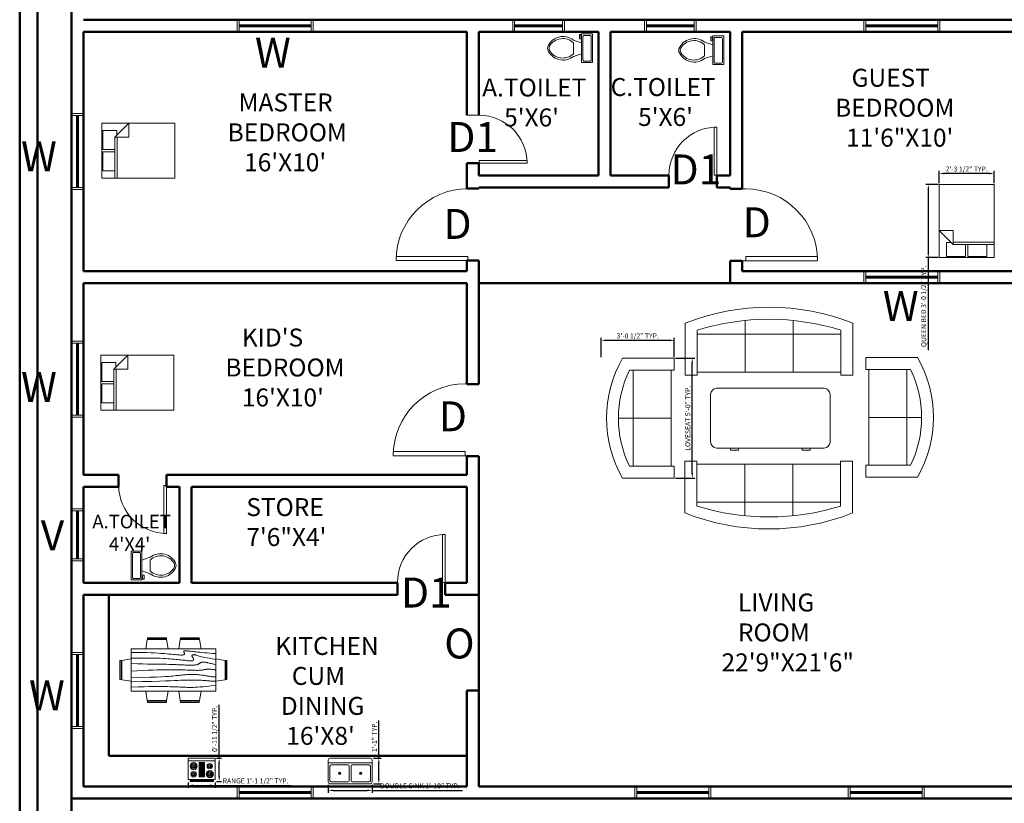
# Model space of a CAD drawing. Units: inches. Extents: x -7040 to -4088, y 6092 to 7645.
# Tile 4 of 11: x -7003 to -6510, y 6471 to 6864. Entities that reach past the tile are written whole.
import ezdxf

# ---------------------------------------------------------------- set-up
doc = ezdxf.new("R2010")
doc.units = ezdxf.units.IN
for name, color, linetype, lineweight in [('A-ANNO-DIMS', 2, 'Continuous', 18), ('A-ANNO-TEXT', 7, 'Continuous', 25), ('A-AREA-IDEN', 3, 'Continuous', 25), ('A-DOOR', 3, 'Continuous', 18), ('A-FLOR-FIXT', 9, 'Continuous', 13), ('A-FURN', 8, 'Continuous', 13), ('A-GLAZ', 4, 'Continuous', 18), ('A-WALL', 7, 'Continuous', 50)]:
    doc.layers.add(name, color=color, linetype=linetype, lineweight=lineweight)
doc.styles.get("Standard").update_dxf_attribs({"font": 'arial.ttf'})
doc.dimstyles.new('ISO-25', dxfattribs={"dimtxt": 2.5, "dimasz": 2.5, "dimexe": 1.25, "dimexo": 0.625, "dimtad": 1, "dimdec": 0, "dimlunit": 3, "dimtxsty": 'Standard', "dimcen": 2.5, "dimadec": 0, "dimazin": 0, "dimtfac": 1, "dimtdec": 0, "dimtmove": 0, "dimatfit": 3, "dimfxl": 1, "dimarcsym": 0})

# ---------------------------------------------------------------- blocks, each defined once
blk = doc.blocks.new('*U8')
for p, q in [((0, 0), (0, -100)), ((750, 0), (750, -100))]:
    blk.add_line(p, q)
blk.add_lwpolyline([(0, 0), (0, 750), (43.75, 750), (43.75, 0)], close=True)
blk.add_arc((0, 0), 750, 0, 90)
blk = doc.blocks.new('Bed - Queen')
for p, q in [((0, -80.00003), (0, 0)), ((0, 0), (59.99999, 0)), ((59.99999, 0), (59.99999, -80.00003)), ((7.99999, -1.2), (28.79998, -1.2)), ((7.99999, -14.4), (7.99999, -1.2)), ((28.79998, -1.2), (28.79998, -14.4)), ((31.19999, -1.2), (51.99999, -1.2)), ((31.19999, -14.4), (31.19999, -1.2)), ((51.99999, -1.2), (51.99999, -16.4)), ((0, -14.4), (44.8, -14.4)), ((44.8, -16.8), (0, -16.8)), ((59.99999, -29.6), (44.8, -14.4)), ((44.8, -14.4), (44.8, -29.6)), ((51.99999, -16.4), (46.79936, -16.4)), ((44.8, -29.6), (59.99999, -29.6)), ((59.99999, -80.00003), (0, -80.00003))]:
    blk.add_line(p, q)
blk = doc.blocks.new('Dining Set - 36 x 72 in.')
for p, q in [((-22.2343, 26.00059), (-23.4847, 17.99762)), ((-22.2304, 26), (-5.7608, 26)), ((-22, 27.5), (-22.1562, 26.50042)), ((-5.8416, 26.5), (-22.1534, 26.5)), ((-22, 27.5), (-6, 27.5)), ((-5.8437, 26.49966), (-6, 27.5)), ((-4.5152, 17.99762), (-5.7655, 25.99926)), ((5.7657, 26.00059), (4.5153, 17.99762)), ((5.7696, 26), (22.2392, 26)), ((6, 27.5), (5.8438, 26.50042)), ((22.1584, 26.5), (5.8466, 26.5)), ((6, 27.5), (22, 27.5)), ((22.1563, 26.49966), (22, 27.5)), ((23.4848, 17.99762), (22.2345, 25.99926)), ((36, 18), (-36, 18)), ((-36, 18), (-36, -18)), ((36, -18), (36, 18)), ((-44.0006, 8.23428), (-35.9976, 9.48474)), ((44.0006, 8.23428), (35.9976, 9.48474)), ((-45.5, 8), (-44.5004, 8.15617)), ((-45.5, 8), (-45.5, -8)), ((-44.5, -8.15843), (-44.5, 8.15338)), ((-44, 8.23041), (-44, -8.23915)), ((44, 8.23041), (44, -8.23915)), ((44.5, -8.15843), (44.5, 8.15338)), ((45.5, 8), (44.5005, 8.15617)), ((45.5, 8), (45.5, -8)), ((-44.4997, -8.15631), (-45.5, -8)), ((-35.9976, -9.48476), (-43.9993, -8.2345)), ((35.9976, -9.48476), (43.9993, -8.2345)), ((44.4997, -8.15631), (45.5, -8)), ((-36, -18), (36, -18)), ((-22.2343, -26.0006), (-23.4847, -17.99762)), ((-4.5152, -17.99762), (-5.7655, -25.99928)), ((5.7657, -26.0006), (4.5153, -17.99762)), ((23.4848, -17.99762), (22.2345, -25.99928)), ((-22.2304, -26), (-5.7608, -26)), ((-22, -27.5), (-22.1562, -26.50044)), ((-5.8416, -26.5), (-22.1534, -26.5)), ((-22, -27.5), (-6, -27.5)), ((-5.8437, -26.49967), (-6, -27.5)), ((5.7696, -26), (22.2392, -26)), ((6, -27.5), (5.8438, -26.50044)), ((22.1584, -26.5), (5.8466, -26.5)), ((6, -27.5), (22, -27.5)), ((22.1563, -26.49967), (22, -27.5))]:
    blk.add_line(p, q)
for points in [[(-36, 15), (-31.1772, 14.97754), (-26.8079, 14.91406), (-22.8538, 14.81543), (-19.276, 14.6875), (-16.0362, 14.53613), (-13.0957, 14.36718), (-10.4159, 14.18652), (-7.9583, 14), (-5.6904, 13.81315), (-3.6035, 13.63021), (-1.6954, 13.45508), (0.0365, 13.29166), (1.5945, 13.14388), (2.9811, 13.01562), (4.1988, 12.9108), (5.25, 12.83333), (6.1393, 12.78613), (6.8802, 12.76823), (7.4883, 12.77767), (7.9792, 12.8125), (8.3685, 12.87077), (8.6719, 12.95052), (8.9049, 13.0498), (9.0833, 13.16666), (9.2205, 13.29899), (9.3216, 13.44401), (9.3895, 13.59879), (9.4271, 13.76041), (9.4373, 13.92594), (9.4232, 14.09245), (9.3875, 14.257), (9.3333, 14.41666), (9.2638, 14.56917), (9.1836, 14.71484), (9.0975, 14.85465), (9.0104, 14.98958), (8.9272, 15.1206), (8.8529, 15.2487), (8.7922, 15.37483), (8.75, 15.5), (8.7305, 15.62467), (8.7344, 15.74739), (8.7617, 15.86621), (8.8125, 15.97916), (8.8867, 16.08431), (8.9844, 16.17968), (9.1055, 16.26334), (9.25, 16.33333), (9.4189, 16.38802), (9.6172, 16.42708), (9.8506, 16.45052), (10.125, 16.45833), (10.4463, 16.45052), (10.8203, 16.42708), (11.2529, 16.38802), (11.75, 16.33333), (12.3184, 16.26318), (12.9694, 16.17838), (13.7151, 16.07991), (14.5677, 15.96875), (15.5395, 15.84586), (16.6426, 15.71224), (17.8893, 15.56884), (19.2917, 15.41666), (20.859, 15.25667), (22.5879, 15.08984), (24.4721, 14.91715), (26.5052, 14.73958), (28.6809, 14.5581), (30.9929, 14.3737), (33.4347, 14.18733), (36, 14)], [(-36, 10), (-28.9766, 10.14274), (-23.1725, 10.20442), (-18.4241, 10.19775), (-14.5677, 10.13541), (-11.4399, 10.03011), (-8.877, 9.89453), (-6.7154, 9.74137), (-4.7917, 9.58333), (-2.9698, 9.43082), (-1.2246, 9.28515), (0.4415, 9.14534), (2.026, 9.01041), (3.5266, 8.87939), (4.9408, 8.7513), (6.266, 8.62516), (7.5, 8.5), (8.6411, 8.37549), (9.6914, 8.2539), (10.6538, 8.13818), (11.5312, 8.03125), (12.3267, 7.93603), (13.043, 7.85547), (13.6831, 7.79248), (14.25, 7.75), (14.7471, 7.7303), (15.1797, 7.73307), (15.5537, 7.75732), (15.875, 7.80208), (16.1494, 7.86637), (16.3828, 7.94922), (16.5811, 8.04964), (16.75, 8.16666), (16.8944, 8.29915), (17.0143, 8.44531), (17.1089, 8.60319), (17.1771, 8.77083), (17.218, 8.94629), (17.2305, 9.1276), (17.2137, 9.31282), (17.1667, 9.5), (17.0895, 9.6875), (16.987, 9.875), (16.8649, 10.0625), (16.7292, 10.25), (16.5856, 10.4375), (16.4401, 10.625), (16.2985, 10.8125), (16.1667, 11), (16.05, 11.18733), (15.9518, 11.3737), (15.8752, 11.5581), (15.8229, 11.73958), (15.798, 11.91715), (15.8034, 12.08984), (15.842, 12.25667), (15.9167, 12.41666), (16.0295, 12.56836), (16.1784, 12.70833), (16.3605, 12.83268), (16.5729, 12.9375), (16.8127, 13.01888), (17.0768, 13.07291), (17.3625, 13.0957), (17.6667, 13.08333), (17.9894, 13.03312), (18.3418, 12.94726), (18.7382, 12.82918), (19.1927, 12.68229), (19.7195, 12.51001), (20.3327, 12.31575), (21.0465, 12.10294), (21.875, 11.875), (22.8357, 11.63354), (23.959, 11.37304), (25.2786, 11.08618), (26.8282, 10.76562), (28.6414, 10.40405), (30.752, 9.99414), (33.1936, 9.52856), (36, 9)], [(-36, 5.5), (-30.7157, 5.3348), (-26.069, 5.20963), (-21.9946, 5.11767), (-18.4271, 5.05208), (-15.3009, 5.00602), (-12.5508, 4.97265), (-10.1112, 4.94515), (-7.9167, 4.91666), (-5.909, 4.88167), (-4.0586, 4.83984), (-2.3429, 4.79215), (-0.7396, 4.73958), (0.7739, 4.6831), (2.22, 4.6237), (3.6213, 4.56233), (5, 4.5), (6.373, 4.43782), (7.7344, 4.3776), (9.0723, 4.32129), (10.375, 4.27083), (11.6309, 4.22819), (12.8281, 4.19531), (13.9551, 4.17415), (15, 4.16666), (15.954, 4.17448), (16.819, 4.19791), (17.6001, 4.23698), (18.3021, 4.29166), (18.9299, 4.36198), (19.4883, 4.44791), (19.9823, 4.54948), (20.4167, 4.66666), (20.7969, 4.79899), (21.1302, 4.94401), (21.4245, 5.09879), (21.6875, 5.26041), (21.9271, 5.42594), (22.1511, 5.59245), (22.3672, 5.757), (22.5834, 5.91666), (22.8065, 6.06868), (23.0404, 6.21093), (23.2879, 6.34147), (23.5521, 6.45833), (23.8358, 6.55957), (24.142, 6.64323), (24.4735, 6.70735), (24.8334, 6.75), (25.2235, 6.76969), (25.642, 6.76692), (26.0858, 6.74267), (26.5521, 6.69791), (27.0379, 6.63362), (27.5404, 6.55078), (28.0565, 6.45036), (28.5834, 6.33333), (29.1242, 6.19987), (29.7071, 6.04687), (30.3661, 5.87044), (31.1354, 5.66666), (32.0493, 5.43164), (33.142, 5.16146), (34.4475, 4.85221), (36, 4.5)], [(-36, -1), (-30.7915, -0.6591), (-26.0195, -0.38216), (-21.6519, -0.16284), (-17.6563, 0.00521), (-14.0005, 0.12833), (-10.6523, 0.21289), (-7.5796, 0.26522), (-4.75, 0.29166), (-2.134, 0.29793), (0.2878, 0.28711), (2.5317, 0.26163), (4.6146, 0.22396), (6.5529, 0.17651), (8.3633, 0.12174), (10.0623, 0.06209), (11.6667, 0), (13.1899, -0.06201), (14.6341, -0.1211), (15.9982, -0.17432), (17.2813, -0.21875), (18.4823, -0.25147), (19.6003, -0.26953), (20.6343, -0.27002), (21.5834, -0.25), (22.4481, -0.20768), (23.2357, -0.14584), (23.9549, -0.06836), (24.6146, 0.02083), (25.2235, 0.11784), (25.7904, 0.21875), (26.3241, 0.31966), (26.8334, 0.41666), (27.3265, 0.50618), (27.8099, 0.58593), (28.2894, 0.65397), (28.7709, 0.70833), (29.2601, 0.74707), (29.763, 0.76823), (30.2855, 0.76985), (30.8334, 0.75), (31.4088, 0.70784), (31.9994, 0.64713), (32.589, 0.57275), (33.1615, 0.48958), (33.7008, 0.4025), (34.1908, 0.3164), (34.6153, 0.23616), (34.9584, 0.16666), (35.2099, 0.11165), (35.3848, 0.07031), (35.504, 0.04069), (35.5886, 0.02083), (35.6594, 0.00879), (35.7377, 0.0026), (35.8442, 0.00032), (36, 0)], [(-36, -6.5), (-27.1843, -6.31267), (-20.084, -6.1263), (-14.469, -5.9419), (-10.1094, -5.76042), (-6.7752, -5.58285), (-4.2363, -5.41016), (-2.2629, -5.24333), (-0.625, -5.08334), (0.8708, -4.93099), (2.2715, -4.78646), (3.5872, -4.64974), (4.8281, -4.52084), (6.0046, -4.39974), (7.127, -4.28646), (8.2053, -4.18099), (9.25, -4.08334), (10.2705, -3.99382), (11.2734, -3.91407), (12.2647, -3.84603), (13.25, -3.79167), (14.2354, -3.75293), (15.2266, -3.73177), (16.2295, -3.73015), (17.25, -3.75), (18.2912, -3.79248), (19.3451, -3.85547), (20.4009, -3.93604), (21.4479, -4.03125), (22.4754, -4.13819), (23.4727, -4.25391), (24.4289, -4.37549), (25.3334, -4.5), (26.1785, -4.62492), (26.9694, -4.74935), (27.7145, -4.87281), (28.4219, -4.99479), (29.1, -5.11483), (29.7572, -5.23242), (30.4016, -5.34709), (31.0417, -5.45834), (31.6837, -5.56437), (32.3262, -5.65821), (32.9658, -5.73153), (33.599, -5.77604), (34.2224, -5.78345), (34.8327, -5.74545), (35.4264, -5.65373), (36, -5.5)], [(-36, -10), (-26.4022, -9.81299), (-18.4675, -9.62891), (-11.9839, -9.45069), (-6.7396, -9.28125), (-2.5226, -9.12354), (0.8789, -8.98047), (3.6769, -8.85498), (6.0833, -8.75), (8.2767, -8.66765), (10.3021, -8.60677), (12.1712, -8.56543), (13.8958, -8.54167), (15.4876, -8.53353), (16.9583, -8.53907), (18.3197, -8.55632), (19.5834, -8.58334), (20.7616, -8.61841), (21.8685, -8.66081), (22.9188, -8.71004), (23.9271, -8.76563), (24.9081, -8.82707), (25.8763, -8.89388), (26.8465, -8.96558), (27.8334, -9.04167), (28.8474, -9.12118), (29.8828, -9.20117), (30.93, -9.27824), (31.9792, -9.34896), (33.0205, -9.40991), (34.0443, -9.45768), (35.0407, -9.48885), (36, -9.5)], [(-36, -14.5), (-30.0881, -14.33513), (-25.0332, -14.21224), (-20.7312, -14.12647), (-17.0781, -14.07292), (-13.97, -14.04671), (-11.3027, -14.04297), (-8.9724, -14.05681), (-6.875, -14.08334), (-4.9224, -14.11833), (-3.0905, -14.16016), (-1.3709, -14.20785), (0.2448, -14.26042), (1.7647, -14.3169), (3.1973, -14.3763), (4.5507, -14.43767), (5.8333, -14.5), (7.0554, -14.5621), (8.235, -14.62175), (9.3922, -14.67652), (10.5469, -14.72396), (11.7192, -14.76164), (12.929, -14.78711), (14.1965, -14.79794), (15.5417, -14.79167), (16.9933, -14.76424), (18.6152, -14.70508), (20.4804, -14.60197), (22.6615, -14.44271), (25.2312, -14.21509), (28.2624, -13.9069), (31.8277, -13.50594), (36, -13)]]:
    blk.add_lwpolyline(points)
blk = doc.blocks.new('Range-Oven - 30 in top')
for p, q in [((0, -3), (30, -3)), ((12, -6), (18, -6)), ((13, -20), (13, -6)), ((14, -6), (14, -20)), ((15, -20), (15, -6)), ((16, -6), (16, -20)), ((17, -20), (17, -6)), ((18, -20), (12, -20)), ((6, -24), (6, -25)), ((8, -25), (8, -24)), ((22, -25), (22, -24)), ((24, -24), (24, -25))]:
    blk.add_line(p, q)
for points in [[(0, -24), (0, 0), (30, 0), (30, -24)], [(12, -21), (12, -5), (18, -5), (18, -21)], [(2, -26), (2, -25), (28, -25), (28, -26)]]:
    blk.add_lwpolyline(points, close=True)
for centre, radius in [((6, -9), 4), ((6, -9), 3), ((6, -9), 2), ((6, -9), 1), ((24, -9), 3), ((24, -9), 2), ((24, -9), 1), ((6, -18), 3), ((6, -18), 2), ((6, -18), 1), ((24, -18), 4), ((24, -18), 3), ((24, -18), 2), ((24, -18), 1)]:
    blk.add_circle(centre, radius)
blk = doc.blocks.new('Sink-double - 36 in top')
for p, q in [((-18, -4), (18, -4)), ((-0.75, -18.5), (-0.75, -6.5)), ((0.75, -6.5), (0.75, -18.5))]:
    blk.add_line(p, q)
for points in [[(-16.5, 0), (16.5, 0)], [(-18, -19.5), (-18, -1.5)], [(-16.5, -18.5), (-16.5, -6.5)], [(-15.5, -5.5), (-1.75, -5.5)], [(1.75, -5.5), (15.5, -5.5)], [(16.5, -6.5), (16.5, -18.5)], [(18, -1.5), (18, -19.5)], [(16.5, -21), (-16.5, -21)], [(-1.75, -19.5), (-15.5, -19.5)], [(15.5, -19.5), (1.75, -19.5)]]:
    blk.add_lwpolyline(points)
for centre, radius in [((-8.5, -12.5), 1), ((-8.5, -12.5), 0.5), ((8.5, -12.5), 1), ((8.5, -12.5), 0.5)]:
    blk.add_circle(centre, radius)
for centre, radius, start, end in [((-16.5, -1.5), 1.5, 90, 180), ((16.5, -1.5), 1.5, 0, 90), ((-15.5, -6.5), 1, 90, 180), ((-1.75, -6.5), 1, 0, 90), ((1.75, -6.5), 1, 90, 180), ((15.5, -6.5), 1, 0, 90), ((-16.5, -19.5), 1.5, 180, 270), ((-15.5, -18.5), 1, 180, 270), ((-1.75, -18.5), 1, 270, 0), ((1.75, -18.5), 1, 180, 270), ((15.5, -18.5), 1, 270, 0), ((16.5, -19.5), 1.5, 270, 0)]:
    blk.add_arc(centre, radius, start, end)
blk = doc.blocks.new('Desk - 30 x 60 in.')
for p, q in [((-26.999995, 0), (26.999995, 0)), ((-29.999995, -27), (-29.999995, -3)), ((29.999995, -3), (29.999995, -27)), ((26.999995, -30), (-26.999995, -30)), ((-20.000005, -30), (-20.000005, -31)), ((-20.000005, -31), (-16.000005, -31)), ((-16.000005, -31), (-16.000005, -30)), ((15.999995, -31), (15.999995, -30)), ((19.999995, -31), (15.999995, -31)), ((19.999995, -30), (19.999995, -31))]:
    blk.add_line(p, q)
for centre, start, end in [((-26.499995, -3.5), 98.1301, 171.8699), ((26.499995, -3.5), 8.130102, 81.8699), ((-26.499995, -26.5), 188.1301, 261.8699), ((26.499995, -26.5), 278.1301, 351.8699)]:
    blk.add_arc(centre, 3.535534, start, end)
blk = doc.blocks.new('Sofa - Roundback 7 ft.')
for p, q in [((-12.00002, -32.4421), (-12.00003, -6.5971)), ((11.99997, -32.4421), (11.99998, -6.5971)), ((-36.000027, -34), (-36.000027, -11.4696)), ((-35.999844, -13.3819), (35.9998, -13.3819)), ((35.99998, -34), (35.99998, -11.4696)), ((-36.000027, -32.4421), (35.99998, -32.4421))]:
    blk.add_line(p, q)
for points in [[(-36.000027, -34), (-42.000027, -34), (-42.000027, -8)], [(41.99998, -8), (41.99998, -34), (35.99998, -34)]]:
    blk.add_lwpolyline(points)
for centre, radius, start, end in [((0, -114.25), 114.25, 68.43141, 111.5686), ((-0.00001, -127.1968), 121.1968, 72.72033, 107.2797)]:
    blk.add_arc(centre, radius, start, end)
blk = doc.blocks.new('Sofa - Roundback Loveseat 5 ft.')
for p, q in [((0, -32.44198), (0, -5.99998)), ((-24, -33.99998), (-24, -11.46958)), ((-23.9998, -13.38178), (23.99986, -13.38178)), ((24.00004, -33.99998), (24.00004, -11.46958)), ((-24, -32.44198), (24.00004, -32.44198))]:
    blk.add_line(p, q)
for points in [[(-24, -33.99998), (-30, -33.99998), (-30, -7.99998)], [(30.00004, -7.99998), (30.00004, -33.99998), (24.00004, -33.99998)]]:
    blk.add_lwpolyline(points)
for centre, radius, start, end in [((0, -60.24998), 60.24998, 60.13715, 119.8628), ((0, -61.38438), 55.38444, 64.32083, 115.6792)]:
    blk.add_arc(centre, radius, start, end)
blk = doc.blocks.new('Toilet - top')
for p, q in [((9.5, -6), (9.5, -2)), ((-10, -8.5), (-8, -8.5)), ((-10, -9.5), (-10, -8.5)), ((-7, -9.5), (-10, -9.5)), ((-8, -8.5), (-8, -8)), ((-7, -8), (-7, -9.5)), ((-4, -8), (-6, -14)), ((4, -14), (-4, -14)), ((4, -8), (6, -14))]:
    blk.add_line(p, q)
blk.add_lwpolyline([(10.5, -8), (10.5, 0), (-10.5, 0), (-10.5, -8)], close=True)
for points in [[(-9.5, -2), (-9.5, -6)], [(8.5, -1), (-8.5, -1)], [(-8.5, -7), (8.5, -7)]]:
    blk.add_lwpolyline(points)
for centre, radius, start, end in [((-8.62, -1.88), 0.884, 81.8699, 188.1301), ((-8.62, -6.12), 0.884, 171.8699, 278.1301), ((8.62, -1.88), 0.884, 351.8699, 98.1301), ((8.62, -6.12), 0.884, 261.8699, 8.1301), ((3.52, -21.58), 12.17, 141.46911, 247.97143), ((4.2, -21.82), 11.33, 136.36773, 238.94682), ((-3.52, -21.58), 12.17, 292.02843, 38.53071), ((-4.2, -21.82), 11.33, 301.05301, 43.63209), ((0, -27.88), 4, 245.73182, 294.26817), ((0, -29), 4, 254.86053, 285.13947)]:
    blk.add_arc(centre, radius, start, end)
blk = doc.blocks.new('WIN-36')
for p, q in [((0, 6), (0, 0)), ((1, 6), (1, 0)), ((37, 6), (37, 0)), ((38, 6), (38, 0)), ((1, 3.5), (37, 3.5)), ((1, 3), (37, 3)), ((1, 2.5), (37, 2.5))]:
    blk.add_line(p, q)
blk = doc.blocks.new('WIN-24')
for p, q in [((0, 6), (0, 0)), ((1, 6), (1, 0)), ((25, 6), (25, 0)), ((26, 6), (26, 0)), ((1, 3.5), (25, 3.5)), ((1, 3), (25, 3)), ((1, 2.5), (25, 2.5))]:
    blk.add_line(p, q)
blk = doc.blocks.new('*D122')
at = {"layer": 'A-ANNO-DIMS', "color": 0, "lineweight": -2, "transparency": 16777216}
for p, q in [((-6542.92, 6781.25), (-6549.04, 6781.25)), ((-6547.79, 6778.75), (-6547.79, 6747.1)), ((-6542.92, 6744.6), (-6549.04, 6744.6)), ((-6547.79, 6744.6), (-6547.79, 6698.25))]:
    blk.add_line(p, q, dxfattribs=at)
at = {"layer": 'A-ANNO-DIMS', "color": 0, "transparency": 16777216}
for points in [[(-6548.2, 6778.75), (-6547.37, 6778.75), (-6547.79, 6781.25)], [(-6548.2, 6747.1), (-6547.37, 6747.1), (-6547.79, 6744.6)]]:
    blk.add_solid(points, dxfattribs=at)
at = {"layer": 'Defpoints', "color": 0, "transparency": 16777216}
for p in [(-6542.29, 6781.25), (-6547.79, 6744.6), (-6542.29, 6744.6)]:
    blk.add_point(p, dxfattribs=at)
at = {"layer": 'A-ANNO-DIMS', "color": 0, "transparency": 16777216, "insert": (-6549.78, 6720.18), "char_height": 2.5, "attachment_point": 5, "rotation": 90}
blk.add_mtext('QUEEN BED 3\'-0 1/2" TYP.', dxfattribs=at)
blk = doc.blocks.new('*D123')
at = {"layer": 'A-ANNO-DIMS', "color": 0, "lineweight": -2, "transparency": 16777216}
for p, q in [((-6542.29, 6781.87), (-6542.29, 6787.99)), ((-6517.31, 6786.74), (-6539.79, 6786.74)), ((-6514.81, 6781.87), (-6514.81, 6787.99))]:
    blk.add_line(p, q, dxfattribs=at)
at = {"layer": 'A-ANNO-DIMS', "color": 0, "transparency": 16777216}
for points in [[(-6539.79, 6787.16), (-6539.79, 6786.33), (-6542.29, 6786.74)], [(-6517.31, 6787.16), (-6517.31, 6786.33), (-6514.81, 6786.74)]]:
    blk.add_solid(points, dxfattribs=at)
at = {"layer": 'Defpoints', "color": 0, "transparency": 16777216}
for p in [(-6542.29, 6786.74), (-6542.29, 6781.25), (-6514.81, 6781.25)]:
    blk.add_point(p, dxfattribs=at)
at = {"layer": 'A-ANNO-DIMS', "color": 0, "transparency": 16777216, "insert": (-6528.55, 6788.66), "char_height": 2.5, "attachment_point": 5}
blk.add_mtext('2\'-3 1/2" TYP.', dxfattribs=at)
blk = doc.blocks.new('*D134')
at = {"layer": 'A-ANNO-DIMS', "color": 0, "lineweight": -2, "transparency": 16777216}
for p, q in [((-6674.42, 6694.16), (-6664.79, 6694.16)), ((-6666.04, 6636.66), (-6666.04, 6691.66)), ((-6674.42, 6634.16), (-6664.79, 6634.16))]:
    blk.add_line(p, q, dxfattribs=at)
at = {"layer": 'A-ANNO-DIMS', "color": 0, "transparency": 16777216}
for points in [[(-6666.46, 6691.66), (-6665.62, 6691.66), (-6666.04, 6694.16)], [(-6666.46, 6636.66), (-6665.62, 6636.66), (-6666.04, 6634.16)]]:
    blk.add_solid(points, dxfattribs=at)
at = {"layer": 'Defpoints', "color": 0, "transparency": 16777216}
for p in [(-6675.04, 6694.16), (-6666.04, 6694.16), (-6675.04, 6634.16)]:
    blk.add_point(p, dxfattribs=at)
at = {"layer": 'A-ANNO-DIMS', "color": 0, "transparency": 16777216, "insert": (-6667.96, 6664.16), "char_height": 2.5, "attachment_point": 5, "rotation": 90}
blk.add_mtext('LOVESEAT 5\'-0" TYP.', dxfattribs=at)
blk = doc.blocks.new('*D135')
at = {"layer": 'A-ANNO-DIMS', "color": 0, "lineweight": -2, "transparency": 16777216}
for p, q in [((-6711.71, 6694.79), (-6711.71, 6704.41)), ((-6675.04, 6694.79), (-6675.04, 6704.41)), ((-6677.54, 6703.16), (-6709.21, 6703.16))]:
    blk.add_line(p, q, dxfattribs=at)
at = {"layer": 'A-ANNO-DIMS', "color": 0, "transparency": 16777216}
for points in [[(-6709.21, 6703.58), (-6709.21, 6702.74), (-6711.71, 6703.16)], [(-6677.54, 6703.58), (-6677.54, 6702.74), (-6675.04, 6703.16)]]:
    blk.add_solid(points, dxfattribs=at)
at = {"layer": 'Defpoints', "color": 0, "transparency": 16777216}
for p in [(-6711.71, 6703.16), (-6711.71, 6694.16), (-6675.04, 6694.16)]:
    blk.add_point(p, dxfattribs=at)
at = {"layer": 'A-ANNO-DIMS', "color": 0, "transparency": 16777216, "insert": (-6693.37, 6705.08), "char_height": 2.5, "attachment_point": 5}
blk.add_mtext('3\'-0 1/2" TYP.', dxfattribs=at)
blk = doc.blocks.new('*D148')
at = {"layer": 'A-ANNO-DIMS', "color": 0, "lineweight": -2, "transparency": 16777216}
for p, q in [((-6918.55, 6481.67), (-6918.55, 6479.03)), ((-6916.05, 6480.28), (-6907.61, 6480.28)), ((-6905.11, 6481.67), (-6905.11, 6479.03)), ((-6905.11, 6480.28), (-6867.04, 6480.28))]:
    blk.add_line(p, q, dxfattribs=at)
at = {"layer": 'A-ANNO-DIMS', "color": 0, "transparency": 16777216}
for points in [[(-6916.05, 6480.69), (-6916.05, 6479.86), (-6918.55, 6480.28)], [(-6907.61, 6480.69), (-6907.61, 6479.86), (-6905.11, 6480.28)]]:
    blk.add_solid(points, dxfattribs=at)
at = {"layer": 'Defpoints', "color": 0, "transparency": 16777216}
for p in [(-6918.55, 6482.29), (-6905.11, 6482.29), (-6905.11, 6480.28)]:
    blk.add_point(p, dxfattribs=at)
at = {"layer": 'A-ANNO-DIMS', "color": 0, "transparency": 16777216, "insert": (-6884.83, 6482.19), "char_height": 2.5, "attachment_point": 5}
blk.add_mtext('RANGE 1\'-1 1/2" TYP.', dxfattribs=at)
blk = doc.blocks.new('*D149')
at = {"layer": 'A-ANNO-DIMS', "color": 0, "lineweight": -2, "transparency": 16777216}
for p, q in [((-6903.1, 6493.94), (-6903.1, 6520.69)), ((-6904.49, 6493.94), (-6901.85, 6493.94)), ((-6903.1, 6484.79), (-6903.1, 6491.44)), ((-6904.49, 6482.29), (-6901.85, 6482.29))]:
    blk.add_line(p, q, dxfattribs=at)
at = {"layer": 'A-ANNO-DIMS', "color": 0, "transparency": 16777216}
for points in [[(-6903.51, 6491.44), (-6902.68, 6491.44), (-6903.1, 6493.94)], [(-6903.51, 6484.79), (-6902.68, 6484.79), (-6903.1, 6482.29)]]:
    blk.add_solid(points, dxfattribs=at)
at = {"layer": 'Defpoints', "color": 0, "transparency": 16777216}
for p in [(-6905.11, 6493.94), (-6903.1, 6493.94), (-6905.11, 6482.29)]:
    blk.add_point(p, dxfattribs=at)
at = {"layer": 'A-ANNO-DIMS', "color": 0, "transparency": 16777216, "insert": (-6905.02, 6508.57), "char_height": 2.5, "attachment_point": 5, "rotation": 90}
blk.add_mtext('0\'-11 1/2" TYP.', dxfattribs=at)
blk = doc.blocks.new('*D154')
at = {"layer": 'A-ANNO-DIMS', "color": 0, "lineweight": -2, "transparency": 16777216}
for p, q in [((-6848.49, 6480.47), (-6848.49, 6476.53)), ((-6845.99, 6477.78), (-6828.92, 6477.78)), ((-6826.42, 6480.47), (-6826.42, 6476.53)), ((-6826.42, 6477.78), (-6781.16, 6477.78))]:
    blk.add_line(p, q, dxfattribs=at)
at = {"layer": 'A-ANNO-DIMS', "color": 0, "transparency": 16777216}
for points in [[(-6845.99, 6478.2), (-6845.99, 6477.37), (-6848.49, 6477.78)], [(-6828.92, 6478.2), (-6828.92, 6477.37), (-6826.42, 6477.78)]]:
    blk.add_solid(points, dxfattribs=at)
at = {"layer": 'Defpoints', "color": 0, "transparency": 16777216}
for p in [(-6848.49, 6481.09), (-6826.42, 6481.09), (-6826.42, 6477.78)]:
    blk.add_point(p, dxfattribs=at)
at = {"layer": 'A-ANNO-DIMS', "color": 0, "transparency": 16777216, "insert": (-6802.54, 6479.7), "char_height": 2.5, "attachment_point": 5}
blk.add_mtext('DOUBLE SINK 1\'-10" TYP.', dxfattribs=at)
blk = doc.blocks.new('*D155')
at = {"layer": 'A-ANNO-DIMS', "color": 0, "lineweight": -2, "transparency": 16777216}
for p, q in [((-6823.11, 6493.97), (-6823.11, 6512.72)), ((-6825.79, 6493.97), (-6821.86, 6493.97)), ((-6823.11, 6483.59), (-6823.11, 6491.47)), ((-6825.79, 6481.09), (-6821.86, 6481.09))]:
    blk.add_line(p, q, dxfattribs=at)
at = {"layer": 'A-ANNO-DIMS', "color": 0, "transparency": 16777216}
for points in [[(-6823.52, 6491.47), (-6822.69, 6491.47), (-6823.11, 6493.97)], [(-6823.52, 6483.59), (-6822.69, 6483.59), (-6823.11, 6481.09)]]:
    blk.add_solid(points, dxfattribs=at)
at = {"layer": 'Defpoints', "color": 0, "transparency": 16777216}
for p in [(-6826.42, 6493.97), (-6823.11, 6493.97), (-6826.42, 6481.09)]:
    blk.add_point(p, dxfattribs=at)
at = {"layer": 'A-ANNO-DIMS', "color": 0, "transparency": 16777216, "insert": (-6824.99, 6504.59), "char_height": 2.5, "attachment_point": 5, "rotation": 90}
blk.add_mtext('1\'-1" TYP.', dxfattribs=at)

msp = doc.modelspace()

# ---------------------------------------------------------------- linework, layer by layer
at = {"layer": 'A-GLAZ'}
for p, q in [((-6977.03, 6816.76), (-6971.03, 6816.76)), ((-6977.03, 6816.76), (-6971.03, 6816.76)), ((-6977.03, 6815.76), (-6971.03, 6815.76)), ((-6977.03, 6815.76), (-6971.03, 6815.76)), ((-6974.53, 6779.76), (-6974.53, 6815.76)), ((-6974.53, 6779.76), (-6974.53, 6815.76)), ((-6974.03, 6779.76), (-6974.03, 6815.76)), ((-6974.03, 6779.76), (-6974.03, 6815.76)), ((-6973.53, 6779.76), (-6973.53, 6815.76)), ((-6973.53, 6779.76), (-6973.53, 6815.76)), ((-6779.03, 6815.91), (-6773.03, 6815.91)), ((-6977.03, 6779.76), (-6971.03, 6779.76)), ((-6977.03, 6779.76), (-6971.03, 6779.76)), ((-6977.03, 6778.76), (-6971.03, 6778.76)), ((-6977.03, 6778.76), (-6971.03, 6778.76)), ((-6977.03, 6702.76), (-6971.03, 6702.76)), ((-6977.03, 6702.76), (-6971.03, 6702.76)), ((-6977.03, 6701.76), (-6971.03, 6701.76)), ((-6977.03, 6701.76), (-6971.03, 6701.76)), ((-6974.53, 6665.76), (-6974.53, 6701.76)), ((-6974.53, 6665.76), (-6974.53, 6701.76)), ((-6974.03, 6665.76), (-6974.03, 6701.76)), ((-6974.03, 6665.76), (-6974.03, 6701.76)), ((-6973.53, 6665.76), (-6973.53, 6701.76)), ((-6973.53, 6665.76), (-6973.53, 6701.76)), ((-6977.03, 6665.76), (-6971.03, 6665.76)), ((-6977.03, 6665.76), (-6971.03, 6665.76)), ((-6977.03, 6664.76), (-6971.03, 6664.76)), ((-6977.03, 6664.76), (-6971.03, 6664.76)), ((-6977.03, 6546.76), (-6971.03, 6546.76)), ((-6977.03, 6546.76), (-6971.03, 6546.76)), ((-6977.03, 6545.76), (-6971.03, 6545.76)), ((-6977.03, 6545.76), (-6971.03, 6545.76)), ((-6974.53, 6509.76), (-6974.53, 6545.76)), ((-6974.53, 6509.76), (-6974.53, 6545.76)), ((-6974.03, 6509.76), (-6974.03, 6545.76)), ((-6974.03, 6509.76), (-6974.03, 6545.76)), ((-6973.53, 6509.76), (-6973.53, 6545.76)), ((-6973.53, 6509.76), (-6973.53, 6545.76)), ((-6977.03, 6509.76), (-6971.03, 6509.76)), ((-6977.03, 6509.76), (-6971.03, 6509.76)), ((-6977.03, 6508.76), (-6971.03, 6508.76)), ((-6977.03, 6508.76), (-6971.03, 6508.76))]:
    msp.add_line(p, q, dxfattribs=at)
at = {"layer": 'A-WALL'}
for p, q in [((-7003.03, 6156.76), (-7003.03, 7513.76)), ((-6994.03, 6179.76), (-6994.03, 7504.76)), ((-6977.03, 6179.76), (-6977.03, 7487.76)), ((-6971.03, 6863.76), (-6475.03, 6863.76)), ((-6971.03, 6857.76), (-6779.03, 6857.76)), ((-6971.03, 6737.76), (-6971.03, 6857.76)), ((-6779.03, 6815.91), (-6779.03, 6857.76)), ((-6773.03, 6857.76), (-6713.03, 6857.76)), ((-6773.03, 6815.91), (-6773.03, 6857.76)), ((-6713.03, 6785.76), (-6713.03, 6857.76)), ((-6707.03, 6785.76), (-6707.03, 6857.76)), ((-6707.03, 6857.76), (-6647.03, 6857.76)), ((-6647.03, 6785.76), (-6647.03, 6857.76)), ((-6641.03, 6857.76), (-6481.03, 6857.76)), ((-6641.03, 6778.99), (-6641.03, 6857.76)), ((-6779.03, 6791.91), (-6773.03, 6791.91)), ((-6779.03, 6779.17), (-6779.03, 6791.91)), ((-6773.03, 6785.76), (-6773.03, 6791.91)), ((-6773.03, 6785.76), (-6713.03, 6785.76)), ((-6707.03, 6785.76), (-6677.73, 6785.76)), ((-6677.73, 6785.76), (-6677.73, 6779.76)), ((-6653.73, 6785.76), (-6653.73, 6779.76)), ((-6653.73, 6785.76), (-6647.03, 6785.76)), ((-6779.03, 6779.17), (-6773.03, 6779.17)), ((-6773.03, 6779.76), (-6677.73, 6779.76)), ((-6773.03, 6779.17), (-6773.03, 6779.76)), ((-6653.73, 6779.76), (-6647.03, 6779.76)), ((-6647.03, 6778.99), (-6647.03, 6779.76)), ((-6647.03, 6778.99), (-6641.03, 6778.99)), ((-6779.03, 6737.76), (-6779.03, 6743.17)), ((-6779.03, 6743.17), (-6773.03, 6743.17)), ((-6773.03, 6681.19), (-6773.03, 6743.17)), ((-6647.03, 6731.76), (-6647.03, 6742.99)), ((-6647.03, 6742.99), (-6641.03, 6742.99)), ((-6641.03, 6737.76), (-6641.03, 6742.99)), ((-6971.03, 6737.76), (-6779.03, 6737.76)), ((-6641.03, 6737.76), (-6481.03, 6737.76)), ((-6971.03, 6731.76), (-6779.03, 6731.76)), ((-6971.03, 6635.76), (-6971.03, 6731.76)), ((-6779.03, 6681.19), (-6779.03, 6731.76)), ((-6773.03, 6731.76), (-6481.03, 6731.76)), ((-6779.03, 6681.19), (-6773.03, 6681.19)), ((-6779.03, 6635.76), (-6779.03, 6645.19)), ((-6779.03, 6645.19), (-6773.03, 6645.19)), ((-6773.03, 6575.76), (-6773.03, 6645.19)), ((-6971.03, 6635.76), (-6953.48, 6635.76)), ((-6953.48, 6629.76), (-6953.48, 6635.76)), ((-6929.48, 6629.76), (-6929.48, 6635.76)), ((-6929.48, 6635.76), (-6779.03, 6635.76)), ((-6971.03, 6629.76), (-6953.48, 6629.76)), ((-6971.03, 6581.76), (-6971.03, 6629.76)), ((-6929.48, 6629.76), (-6923.03, 6629.76)), ((-6923.03, 6581.76), (-6923.03, 6629.76)), ((-6917.03, 6581.76), (-6917.03, 6629.76)), ((-6917.03, 6629.76), (-6779.03, 6629.76)), ((-6779.03, 6581.76), (-6779.03, 6629.76)), ((-6971.03, 6581.76), (-6923.03, 6581.76)), ((-6917.03, 6581.76), (-6813.77, 6581.76)), ((-6813.77, 6581.76), (-6813.77, 6575.76)), ((-6789.77, 6581.76), (-6789.77, 6575.76)), ((-6789.77, 6581.76), (-6779.03, 6581.76)), ((-6971.03, 6575.76), (-6813.77, 6575.76)), ((-6971.03, 6479.76), (-6971.03, 6575.76)), ((-6958.39, 6575.76), (-6958.39, 6495.11)), ((-6789.77, 6575.76), (-6773.03, 6575.76)), ((-6773.03, 6527.76), (-6773.03, 6575.76)), ((-6779.03, 6479.76), (-6779.03, 6527.76)), ((-6779.03, 6527.76), (-6773.03, 6527.76)), ((-6773.03, 6479.76), (-6773.03, 6527.76)), ((-6958.39, 6495.11), (-6779.03, 6495.11)), ((-6971.03, 6479.76), (-6779.03, 6479.76)), ((-6773.03, 6479.76), (-6481.03, 6479.76)), ((-6977.03, 6473.76), (-6475.03, 6473.76))]:
    msp.add_line(p, q, dxfattribs=at)

# ---------------------------------------------------------------- block references
at = {"layer": 'A-DOOR'}
for p, xscale, yscale, zscale, rotation in [((-6772.83, 6791.91), -0.0319999973918968, 0.0319999973918968, 0.0319999973918968, 270), ((-6778.48, 6743.1), 0.0480047089255457, 0.0480047089255457, 0.0480047089255457, 90), ((-6639.23, 6742.99), -0.0479999965272596, 0.0479999965272596, 0.0479999965272596, 270), ((-6779.87, 6645.4), 0.0480047089255457, 0.0480047089255457, 0.0480047089255457, 90), ((-6929.42, 6630.48), 0.0320007809907896, 0.0320007809907896, 0.0320007809907896, 180)]:
    msp.add_blockref('*U8', p, dxfattribs=dict(at, xscale=xscale, yscale=yscale, zscale=zscale, rotation=rotation))
for p, xscale, yscale, zscale in [((-6653.73, 6785.96), -0.0319999999999955, 0.0319999999999955, 0.0319999999999955), ((-6789.77, 6581.96), -0.0319999954706333, 0.0319999954706333, 0.0319999954706333)]:
    msp.add_blockref('*U8', p, dxfattribs=dict(at, xscale=xscale, yscale=yscale, zscale=zscale))
at = {"layer": 'A-FLOR-FIXT', "xscale": 0.6837915443005316, "yscale": 0.6837915443005316, "zscale": 0.6837915443005316}
for p, rotation in [((-6716.01, 6849.43), 270), ((-6650.28, 6848.42), 270), ((-6947.23, 6590.41), 89.99999999999999)]:
    msp.add_blockref('Toilet - top', p, dxfattribs=dict(at, rotation=rotation))
at = {"layer": 'A-FLOR-FIXT'}
for name, p, xscale, yscale, zscale in [('Range-Oven - 30 in top', (-6918.55, 6493.94), 0.4479334271382261, 0.4479334271382261, 0.4479334271382261), ('Sink-double - 36 in top', (-6837.45, 6493.97), 0.6130704979608608, 0.6130704979608608, 0.6130704979608608)]:
    msp.add_blockref(name, p, dxfattribs=dict(at, xscale=xscale, yscale=yscale, zscale=zscale))
at = {"layer": 'A-FURN', "xscale": 0.4580400962997241, "yscale": 0.4580400962997241, "zscale": 0.4580400962997241}
for p, rotation in [((-6961.93, 6784.43), 90), ((-6514.81, 6744.6), 180), ((-6962.41, 6668.19), 90)]:
    msp.add_blockref('Bed - Queen', p, dxfattribs=dict(at, rotation=rotation))
at = {"layer": 'A-FURN'}
for name, p in [('Sofa - Roundback 7 ft.', (-6627.57, 6719.72)), ('Desk - 30 x 60 in.', (-6626.93, 6679.19))]:
    msp.add_blockref(name, p, dxfattribs=at)
for name, p, rotation in [('Sofa - Roundback Loveseat 5 ft.', (-6545.15, 6664.59), 270), ('Sofa - Roundback Loveseat 5 ft.', (-6709.04, 6664.16), 89.99999999999999), ('Sofa - Roundback 7 ft.', (-6627.71, 6608.72), 180)]:
    msp.add_blockref(name, p, dxfattribs=dict(at, rotation=rotation))
at = {"layer": 'A-FURN', "xscale": 0.5884256662281149, "yscale": 0.5884256662281149, "zscale": 0.5884256662281149}
msp.add_blockref('Dining Set - 36 x 72 in.', (-6926, 6538.05), dxfattribs=at)
at = {"layer": 'A-GLAZ'}
for p in [(-6894.03, 6857.76), (-6580.03, 6857.76), (-6580.03, 6731.76), (-6894.03, 6473.76), (-6694.76, 6473.76), (-6587.87, 6473.76)]:
    msp.add_blockref('WIN-36', p, dxfattribs=at)
for p, rotation in [((-6730.03, 6863.76), 180), ((-6664.03, 6863.76), 180), ((-6977.03, 6618.76), 269.999999999997)]:
    msp.add_blockref('WIN-24', p, dxfattribs=dict(at, rotation=rotation))

# ---------------------------------------------------------------- texts
at = {"layer": 'A-ANNO-TEXT', "char_height": 15, "attachment_point": 1}
for s, insert in [('{W}', (-6885.16, 6854.68)), ('{D1}', (-6788.77, 6812.5)), ('{W}', (-7002.38, 6802.78)), ('{D1}', (-6676.91, 6796.26)), ('{D}', (-6790.69, 6768.97)), ('{D}', (-6640.78, 6769.79)), ('{W}', (-6570.58, 6727.92)), ('{W}', (-7002.38, 6687.3)), ('{D}', (-6792.99, 6672.61)), ('{V}', (-6992.5, 6613.06)), ('{D1}', (-6811.98, 6584.35)), ('{O}', (-6790.3, 6558.85)), ('{W}', (-6998.39, 6532.87))]:
    msp.add_mtext_dynamic_manual_height_columns(s, width=701.5203, gutter_width=12.5, heights=[0], dxfattribs=dict(at, insert=insert))
at = {"layer": 'A-AREA-IDEN', "attachment_point": 1}
for s, insert, char_height in [('{   GUEST\\PBEDROOM\\P  11\'6"X10\'}', (-6594.47, 6839.18), 9), ("{  A.TOILET\\P      5'X6'}", (-6776.81, 6834.3), 9), ("{  C.TOILET\\P       5'X6'}", (-6712.43, 6834.54), 9), ("{  MASTER\\PBEDROOM\\P   16'X10'}", (-6898.84, 6826.83), 9), ("{   KID'S\\PBEDROOM\\P   16'X10'}", (-6899.98, 6709.07), 9), ('{STORE\\P7\'6"X4\'}', (-6889.48, 6624.15), 9), ("{A.TOILET\\P    4'X4'}", (-6966.62, 6615.8), 6.782), ('{    LIVING\\P    ROOM\\P 22\'9"X21\'6"}', (-6654.16, 6576.38), 9), ("{KITCHEN\\P   CUM\\P DINING\\P  16'X8'}", (-6874.94, 6554.6), 9)]:
    msp.add_mtext_dynamic_manual_height_columns(s, width=930.9751, gutter_width=12.5, heights=[0], dxfattribs=dict(at, insert=insert, char_height=char_height))

# ---------------------------------------------------------------- dimensions: what is measured, and where the dimension line sits
at = {"layer": 'A-ANNO-DIMS'}
for base, p1, p2, angle, text, picture, middle in [((-6542.29, 6786.74), (-6514.81, 6781.25), (-6542.29, 6781.25), 180, '<> TYP.', '*D123', (-6528.55, 6788.66)), ((-6547.7879, 6744.6022), (-6542.2914, 6781.2454), (-6542.2914, 6744.6022), 270, 'QUEEN BED <> TYP.', '*D122', (-6549.7823, 6720.1769)), ((-6711.71, 6703.16), (-6675.04, 6694.16), (-6711.71, 6694.16), 180, '<> TYP.', '*D135', (-6693.37, 6705.08)), ((-6666.04, 6694.16), (-6675.04, 6634.16), (-6675.04, 6694.16), 90, 'LOVESEAT <> TYP.', '*D134', (-6667.96, 6664.16)), ((-6903.0974, 6493.938), (-6905.1131, 6482.2918), (-6905.1131, 6493.938), 90, '<> TYP.', '*D149', (-6905.015, 6508.5663)), ((-6823.11, 6493.97), (-6826.42, 6481.09), (-6826.42, 6493.97), 90, '<> TYP.', '*D155', (-6824.99, 6504.59))]:
    dim = msp.add_linear_dim(base=base, p1=p1, p2=p2, angle=angle, text=text, dimstyle='ISO-25', override={"dimdec": 1, "dimrnd": 0, "dimzin": 1, "dimlunit": 4, "dimfrac": 2}, dxfattribs=at)
    dim.commit()
    dim.dimension.update_dxf_attribs({"geometry": picture, "text_midpoint": middle})
for base, p1, p2, text, picture, middle in [((-6905.11, 6480.28), (-6918.55, 6482.29), (-6905.11, 6482.29), 'RANGE <> TYP.', '*D148', (-6884.83, 6482.19)), ((-6826.42, 6477.78), (-6848.49, 6481.09), (-6826.42, 6481.09), 'DOUBLE SINK <> TYP.', '*D154', (-6802.54, 6479.7))]:
    dim = msp.add_linear_dim(base=base, p1=p1, p2=p2, text=text, dimstyle='ISO-25', override={"dimdec": 1, "dimrnd": 0, "dimzin": 1, "dimlunit": 4, "dimfrac": 2}, dxfattribs=at)
    dim.commit()
    dim.dimension.update_dxf_attribs({"geometry": picture, "text_midpoint": middle})

doc.saveas('drawing.dxf')
